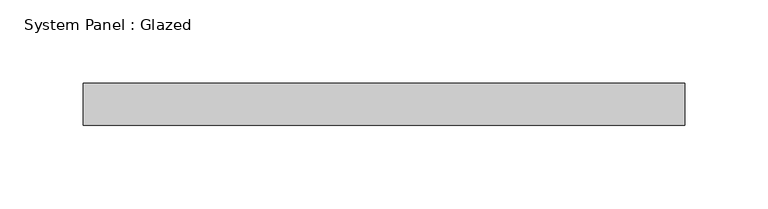
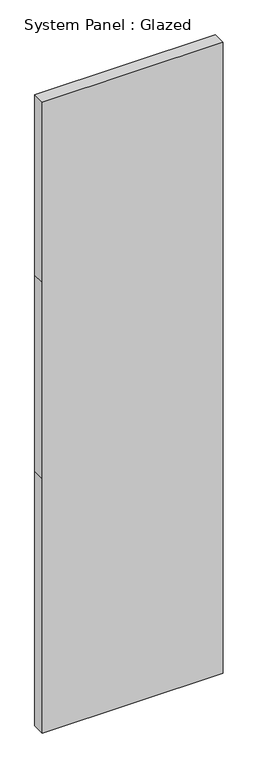
"""IFC4 building model written with IfcOpenShell, lengths in millimetres: plate geometry, System Panel : Glazed."""

from ifc_helpers import new_model, si_unit, frame, origin, place, context, project, spatial, polyline, outline, extrude, source, transform, mapped, element, save


def system_panel_glazed_fdb755d2(model_context):
    return source(origin(), model_context, "Body", "SweptSolid", [
        extrude(outline(polyline([(0.0, -180.975), (0.0, 180.975), (537.6333333, 180.975), (952.5, 180.975), (1333.7313568, 180.975), (1333.7313568, -180.975), (952.5, -180.975), (537.6333333, -180.975), (0.0, -180.975)])), frame((0.0, 19.05, 0.0), z_axis=(0.0, 1.0, 0.0), x_axis=(0.0, 0.0, 1.0)), (0.0, 0.0, 1.0), 25.4),
    ])


if __name__ == "__main__":
    model = new_model("IFC4")
    model_context = context("Model", 3, world=origin())
    ifc_project = project(units=[si_unit("LENGTHUNIT", "METRE", prefix="MILLI")], contexts=[model_context])
    site = spatial("IfcSite", under=ifc_project)
    building = spatial("IfcBuilding", under=site)
    placement = place(None, origin())
    system_panel_glazed_shape = system_panel_glazed_fdb755d2(model_context)
    element("IfcPlate", 1, ObjectType="System Panel : Glazed", at=placement, inside=building, context=model_context, shape_type="MappedRepresentation", body=[
        mapped(system_panel_glazed_shape, transform((0.0, 0.0, 0.0), x_axis=(1.0, 0.0, 0.0), y_axis=(0.0, 1.0, 0.0), z_axis=(0.0, 0.0, 1.0))),
    ])
    save(model, "model.ifc")

# Revit data of these elements
# Type "System Panel : Glazed"
#   Construction Type Id = "GSP4R"
#   Analytic Construction = "1/8 in Pilkington single glazing"
#   Visual Light Transmittance = 0.9
#   Solar Heat Gain Coefficient = 0.86
#   Heat Transfer Coefficient (U) = 1.18115 BTU/(h·ft²·°F)
#   Define Thermal Properties by = 1
# Element 1 (IfcPlate, "System Panel : Glazed")
#   Materials on its faces: "Glass"
# Materials
#   "Glass": class "Glass", colour RGB 0 128 192, transparency 0.75, Description = "Soda Lime Glass", Cost = 0
